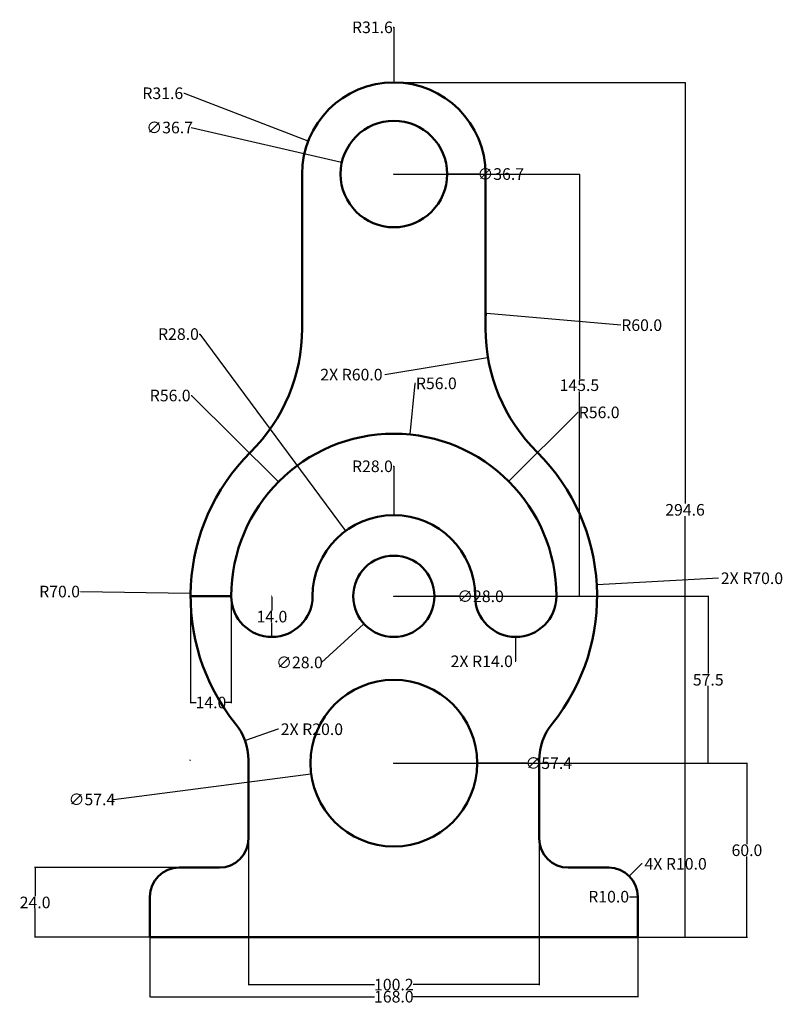
# Model space of a CAD drawing. Units: inches. Extents: x -29 to 234, y -38 to 302.
import ezdxf

# ---------------------------------------------------------------- set-up
doc = ezdxf.new("R2010")
doc.units = ezdxf.units.IN
doc.header["$MEASUREMENT"] = 0
doc.layers.add('M-DIMS', color=2, linetype='Continuous', lineweight=25)
doc.layers.add('M-OUTL', color=7, linetype='Continuous', lineweight=50)
doc.styles.get("Standard").update_dxf_attribs({"font": 'arial.ttf'})
doc.dimstyles.get("Standard").update_dxf_attribs({"dimtxt": 4, "dimasz": 0.18, "dimexe": 0.18, "dimexo": 0.0625, "dimgap": 0.09, "dimtad": 0, "dimtih": 1, "dimtoh": 1, "dimdec": 1, "dimzin": 0, "dimdsep": 46, "dimtxsty": 'Standard', "dimcen": 0.09, "dimadec": 0, "dimazin": 0, "dimtfac": 1, "dimtdec": 1, "dimtofl": 0, "dimtmove": 0, "dimatfit": 3, "dimfxl": 1, "dimtolj": 1, "dimtzin": 0, "dimarcsym": 0})

# ---------------------------------------------------------------- blocks, each defined once
blk = doc.blocks.new('*D1')
at = {"layer": 'Defpoints', "color": 0, "transparency": 16777216}
for p in [(100.04, 45.32), (100.04, -14.68), (221.66, -14.68)]:
    blk.add_point(p, dxfattribs=at)
at = {"layer": 'M-DIMS', "color": 0, "lineweight": -2, "transparency": 16777216}
for p, q in [((100.1, 45.32), (221.84, 45.32)), ((221.66, 45.14), (221.66, 17.46)), ((221.66, -14.5), (221.66, 13.19)), ((100.1, -14.68), (221.84, -14.68))]:
    blk.add_line(p, q, dxfattribs=at)
at = {"layer": 'M-DIMS', "color": 0, "transparency": 16777216}
for points in [[(221.63, 45.14), (221.69, 45.14), (221.66, 45.32)], [(221.63, -14.5), (221.69, -14.5), (221.66, -14.68)]]:
    blk.add_solid(points, dxfattribs=at)
at = {"layer": 'M-DIMS', "color": 0, "transparency": 16777216, "insert": (221.66, 15.32), "char_height": 4, "attachment_point": 5}
blk.add_mtext('\\A1;60.0', dxfattribs=at)
blk = doc.blocks.new('*D2')
at = {"layer": 'Defpoints', "color": 0, "transparency": 16777216}
for p in [(100.04, 102.82), (100.04, 45.32), (208.33, 45.32)]:
    blk.add_point(p, dxfattribs=at)
at = {"layer": 'M-DIMS', "color": 0, "lineweight": -2, "transparency": 16777216}
for p, q in [((100.1, 102.82), (208.51, 102.82)), ((208.33, 102.64), (208.33, 76.2)), ((208.33, 45.5), (208.33, 71.95)), ((100.1, 45.32), (208.51, 45.32))]:
    blk.add_line(p, q, dxfattribs=at)
at = {"layer": 'M-DIMS', "color": 0, "transparency": 16777216}
for points in [[(208.3, 102.64), (208.36, 102.64), (208.33, 102.82)], [(208.3, 45.5), (208.36, 45.5), (208.33, 45.32)]]:
    blk.add_solid(points, dxfattribs=at)
at = {"layer": 'M-DIMS', "color": 0, "transparency": 16777216, "insert": (208.33, 74.07), "char_height": 4, "attachment_point": 5}
blk.add_mtext('\\A1;57.5', dxfattribs=at)
blk = doc.blocks.new('*D3')
at = {"layer": 'Defpoints', "color": 0, "transparency": 16777216}
for p in [(100.04, 248.32), (100.04, 102.82), (163.95, 102.82)]:
    blk.add_point(p, dxfattribs=at)
at = {"layer": 'M-DIMS', "color": 0, "lineweight": -2, "transparency": 16777216}
for p, q in [((100.1, 248.32), (164.13, 248.32)), ((163.95, 248.14), (163.95, 177.71)), ((163.95, 103), (163.95, 173.44)), ((100.1, 102.82), (164.13, 102.82))]:
    blk.add_line(p, q, dxfattribs=at)
at = {"layer": 'M-DIMS', "color": 0, "transparency": 16777216}
for points in [[(163.92, 248.14), (163.98, 248.14), (163.95, 248.32)], [(163.92, 103), (163.98, 103), (163.95, 102.82)]]:
    blk.add_solid(points, dxfattribs=at)
at = {"layer": 'M-DIMS', "color": 0, "transparency": 16777216, "insert": (163.95, 175.57), "char_height": 4, "attachment_point": 5}
blk.add_mtext('\\A1;145.5', dxfattribs=at)
blk = doc.blocks.new('*D4')
at = {"layer": 'Defpoints', "color": 0, "transparency": 16777216}
for p in [(128.5, 49.01), (71.57, 41.64)]:
    blk.add_point(p, dxfattribs=at)
at = {"layer": 'M-DIMS', "color": 0, "lineweight": -2, "transparency": 16777216}
for p, q in [((99.95, 45.32), (100.13, 45.32)), ((100.04, 45.23), (100.04, 45.41)), ((3.49, 32.83), (71.4, 41.62))]:
    blk.add_line(p, q, dxfattribs=at)
at = {"layer": 'M-DIMS', "color": 0, "transparency": 16777216}
blk.add_solid([(71.39, 41.65), (71.4, 41.59), (71.57, 41.64)], dxfattribs=at)
at = {"layer": 'M-DIMS', "color": 0, "transparency": 16777216, "insert": (-3.96, 32.83), "char_height": 4, "attachment_point": 5}
blk.add_mtext('\\A1;∅57.4', dxfattribs=at)
blk = doc.blocks.new('*D5')
at = {"layer": 'Defpoints', "color": 0, "transparency": 16777216}
for p in [(60.3, 142.29), (100.04, 102.82)]:
    blk.add_point(p, dxfattribs=at)
at = {"layer": 'M-DIMS', "color": 0, "lineweight": -2, "transparency": 16777216}
for p, q in [((30.19, 172.01), (30.37, 172.01)), ((30.37, 172.01), (60.18, 142.41)), ((99.95, 102.82), (100.13, 102.82)), ((100.04, 102.73), (100.04, 102.91))]:
    blk.add_line(p, q, dxfattribs=at)
at = {"layer": 'M-DIMS', "color": 0, "transparency": 16777216}
blk.add_solid([(60.2, 142.44), (60.16, 142.39), (60.3, 142.29)], dxfattribs=at)
at = {"layer": 'M-DIMS', "color": 0, "transparency": 16777216, "insert": (23, 172.01), "char_height": 4, "attachment_point": 5}
blk.add_mtext('\\A1;R56.0', dxfattribs=at)
blk = doc.blocks.new('*D6')
at = {"layer": 'Defpoints', "color": 0, "transparency": 16777216}
for p in [(83.39, 125.34), (100.04, 102.82)]:
    blk.add_point(p, dxfattribs=at)
at = {"layer": 'M-DIMS', "color": 0, "lineweight": -2, "transparency": 16777216}
for p, q in [((33.04, 193.18), (33.22, 193.18)), ((33.22, 193.18), (83.28, 125.48)), ((99.95, 102.82), (100.13, 102.82)), ((100.04, 102.73), (100.04, 102.91))]:
    blk.add_line(p, q, dxfattribs=at)
at = {"layer": 'M-DIMS', "color": 0, "transparency": 16777216}
blk.add_solid([(83.31, 125.5), (83.26, 125.46), (83.39, 125.34)], dxfattribs=at)
at = {"layer": 'M-DIMS', "color": 0, "transparency": 16777216, "insert": (25.85, 193.18), "char_height": 4, "attachment_point": 5}
blk.add_mtext('\\A1;R28.0', dxfattribs=at)
blk = doc.blocks.new('*D7')
at = {"layer": 'Defpoints', "color": 0, "transparency": 16777216}
for p in [(58.04, 102.82), (58.04, 88.82), (58.04, 88.82)]:
    blk.add_point(p, dxfattribs=at)
at = {"layer": 'M-DIMS', "color": 0, "lineweight": -2, "transparency": 16777216}
for p, q in [((57.97, 102.82), (57.86, 102.82)), ((58.04, 102.64), (58.04, 97.96)), ((58.04, 89), (58.04, 93.69)), ((57.97, 88.82), (57.86, 88.82))]:
    blk.add_line(p, q, dxfattribs=at)
at = {"layer": 'M-DIMS', "color": 0, "transparency": 16777216}
for points in [[(58.01, 102.64), (58.07, 102.64), (58.04, 102.82)], [(58.01, 89), (58.07, 89), (58.04, 88.82)]]:
    blk.add_solid(points, dxfattribs=at)
at = {"layer": 'M-DIMS', "color": 0, "transparency": 16777216, "insert": (58.04, 95.82), "char_height": 4, "attachment_point": 5}
blk.add_mtext('\\A1;14.0', dxfattribs=at)
blk = doc.blocks.new('*D8')
at = {"layer": 'Defpoints', "color": 0, "transparency": 16777216}
for p in [(110.36, 112.28), (89.72, 93.37)]:
    blk.add_point(p, dxfattribs=at)
at = {"layer": 'M-DIMS', "color": 0, "lineweight": -2, "transparency": 16777216}
for p, q in [((99.95, 102.82), (100.13, 102.82)), ((100.04, 102.73), (100.04, 102.91)), ((75.17, 80.04), (89.58, 93.24)), ((74.99, 80.04), (75.17, 80.04))]:
    blk.add_line(p, q, dxfattribs=at)
at = {"layer": 'M-DIMS', "color": 0, "transparency": 16777216}
blk.add_solid([(89.56, 93.27), (89.6, 93.22), (89.72, 93.37)], dxfattribs=at)
at = {"layer": 'M-DIMS', "color": 0, "transparency": 16777216, "insert": (67.54, 80.04), "char_height": 4, "attachment_point": 5}
blk.add_mtext('\\A1;∅28.0', dxfattribs=at)
blk = doc.blocks.new('*D9')
at = {"layer": 'Defpoints', "color": 0, "transparency": 16777216}
for p in [(30.05, 103.88), (100.04, 102.82)]:
    blk.add_point(p, dxfattribs=at)
at = {"layer": 'M-DIMS', "color": 0, "lineweight": -2, "transparency": 16777216}
for p, q in [((-7.91, 104.46), (29.87, 103.89)), ((99.95, 102.82), (100.13, 102.82)), ((100.04, 102.73), (100.04, 102.91))]:
    blk.add_line(p, q, dxfattribs=at)
at = {"layer": 'M-DIMS', "color": 0, "transparency": 16777216}
blk.add_solid([(29.87, 103.92), (29.86, 103.86), (30.05, 103.88)], dxfattribs=at)
at = {"layer": 'M-DIMS', "color": 0, "transparency": 16777216, "insert": (-15.1, 104.46), "char_height": 4, "attachment_point": 5}
blk.add_mtext('\\A1;R70.0', dxfattribs=at)
blk = doc.blocks.new('*D10')
at = {"layer": 'Defpoints', "color": 0, "transparency": 16777216}
for p in [(82.15, 252.43), (117.92, 244.21)]:
    blk.add_point(p, dxfattribs=at)
at = {"layer": 'M-DIMS', "color": 0, "lineweight": -2, "transparency": 16777216}
for p, q in [((30.28, 264.35), (81.98, 252.47)), ((99.95, 248.32), (100.13, 248.32)), ((100.04, 248.23), (100.04, 248.41))]:
    blk.add_line(p, q, dxfattribs=at)
at = {"layer": 'M-DIMS', "color": 0, "transparency": 16777216}
blk.add_solid([(81.98, 252.5), (81.97, 252.44), (82.15, 252.43)], dxfattribs=at)
at = {"layer": 'M-DIMS', "color": 0, "transparency": 16777216, "insert": (22.82, 264.35), "char_height": 4, "attachment_point": 5}
blk.add_mtext('\\A1;∅36.7', dxfattribs=at)
blk = doc.blocks.new('*D11')
at = {"layer": 'Defpoints', "color": 0, "transparency": 16777216}
for p in [(70.55, 259.69), (100.04, 248.32)]:
    blk.add_point(p, dxfattribs=at)
at = {"layer": 'M-DIMS', "color": 0, "lineweight": -2, "transparency": 16777216}
for p, q in [((27.65, 276.16), (27.83, 276.16)), ((27.83, 276.16), (70.39, 259.76)), ((99.95, 248.32), (100.13, 248.32)), ((100.04, 248.23), (100.04, 248.41))]:
    blk.add_line(p, q, dxfattribs=at)
at = {"layer": 'M-DIMS', "color": 0, "transparency": 16777216}
blk.add_solid([(70.4, 259.79), (70.37, 259.73), (70.55, 259.69)], dxfattribs=at)
at = {"layer": 'M-DIMS', "color": 0, "transparency": 16777216, "insert": (20.46, 276.16), "char_height": 4, "attachment_point": 5}
blk.add_mtext('\\A1;R31.6', dxfattribs=at)
blk = doc.blocks.new('*D12')
at = {"layer": 'Defpoints', "color": 0, "transparency": 16777216}
for p in [(131.87, 200.31), (191.64, 195.07)]:
    blk.add_point(p, dxfattribs=at)
at = {"layer": 'M-DIMS', "color": 0, "lineweight": -2, "transparency": 16777216}
blk.add_line((178.22, 196.25), (132.05, 200.29), dxfattribs=at)
blk.add_arc((191.64, 195.07), 60, 174.821, 179.9403, dxfattribs=at)
at = {"layer": 'M-DIMS', "color": 0, "transparency": 16777216}
blk.add_solid([(132.05, 200.32), (132.04, 200.26), (131.87, 200.31)], dxfattribs=at)
at = {"layer": 'M-DIMS', "color": 0, "transparency": 16777216, "insert": (185.41, 196.25), "char_height": 4, "attachment_point": 5}
blk.add_mtext('\\A1;R60.0', dxfattribs=at)
blk = doc.blocks.new('*D13')
at = {"layer": 'Defpoints', "color": 0, "transparency": 16777216}
for p in [(16.04, -14.68), (184.04, -14.68), (184.04, -35.15)]:
    blk.add_point(p, dxfattribs=at)
at = {"layer": 'M-DIMS', "color": 0, "lineweight": -2, "transparency": 16777216}
for p, q in [((16.04, -14.74), (16.04, -35.33)), ((184.04, -14.74), (184.04, -35.33)), ((16.22, -35.15), (93.39, -35.15)), ((183.86, -35.15), (106.68, -35.15))]:
    blk.add_line(p, q, dxfattribs=at)
at = {"layer": 'M-DIMS', "color": 0, "transparency": 16777216}
for points in [[(16.22, -35.12), (16.22, -35.18), (16.04, -35.15)], [(183.86, -35.12), (183.86, -35.18), (184.04, -35.15)]]:
    blk.add_solid(points, dxfattribs=at)
at = {"layer": 'M-DIMS', "color": 0, "transparency": 16777216, "insert": (100.04, -35.15), "char_height": 4, "attachment_point": 5}
blk.add_mtext('\\A1;168.0', dxfattribs=at)
blk = doc.blocks.new('*D14')
at = {"layer": 'Defpoints', "color": 0, "transparency": 16777216}
for p in [(32.99, 9.32), (-23.53, -14.68), (16.04, -14.68)]:
    blk.add_point(p, dxfattribs=at)
at = {"layer": 'M-DIMS', "color": 0, "lineweight": -2, "transparency": 16777216}
for p, q in [((32.92, 9.32), (-23.71, 9.32)), ((-23.53, 9.14), (-23.53, -0.54)), ((-23.53, -14.5), (-23.53, -4.81)), ((15.97, -14.68), (-23.71, -14.68))]:
    blk.add_line(p, q, dxfattribs=at)
at = {"layer": 'M-DIMS', "color": 0, "transparency": 16777216}
for points in [[(-23.56, 9.14), (-23.5, 9.14), (-23.53, 9.32)], [(-23.56, -14.5), (-23.5, -14.5), (-23.53, -14.68)]]:
    blk.add_solid(points, dxfattribs=at)
at = {"layer": 'M-DIMS', "color": 0, "transparency": 16777216, "insert": (-23.53, -2.68), "char_height": 4, "attachment_point": 5}
blk.add_mtext('\\A1;24.0', dxfattribs=at)
blk = doc.blocks.new('*D15')
at = {"layer": 'Defpoints', "color": 0, "transparency": 16777216}
for p in [(174.04, -0.68), (184.04, -0.68)]:
    blk.add_point(p, dxfattribs=at)
at = {"layer": 'M-DIMS', "color": 0, "lineweight": -2, "transparency": 16777216}
blk.add_line((181.23, -0.68), (183.86, -0.68), dxfattribs=at)
blk.add_arc((174.04, -0.68), 10, 358.9687, 359.6419, dxfattribs=at)
at = {"layer": 'M-DIMS', "color": 0, "transparency": 16777216}
blk.add_solid([(183.86, -0.65), (183.86, -0.71), (184.04, -0.68)], dxfattribs=at)
at = {"layer": 'M-DIMS', "color": 0, "transparency": 16777216, "insert": (174.04, -0.68), "char_height": 4, "attachment_point": 5}
blk.add_mtext('\\A1;R10.0', dxfattribs=at)
blk = doc.blocks.new('*D16')
at = {"layer": 'Defpoints', "color": 0, "transparency": 16777216}
for p in [(105.55, 158.55), (100.04, 102.82)]:
    blk.add_point(p, dxfattribs=at)
at = {"layer": 'M-DIMS', "color": 0, "lineweight": -2, "transparency": 16777216}
for p, q in [((107.3, 176.19), (105.57, 158.73)), ((107.48, 176.19), (107.3, 176.19)), ((99.95, 102.82), (100.13, 102.82)), ((100.04, 102.73), (100.04, 102.91))]:
    blk.add_line(p, q, dxfattribs=at)
at = {"layer": 'M-DIMS', "color": 0, "transparency": 16777216}
blk.add_solid([(105.54, 158.73), (105.6, 158.73), (105.55, 158.55)], dxfattribs=at)
at = {"layer": 'M-DIMS', "color": 0, "transparency": 16777216, "insert": (114.67, 176.19), "char_height": 4, "attachment_point": 5}
blk.add_mtext('\\A1;R56.0', dxfattribs=at)
blk = doc.blocks.new('*D17')
at = {"layer": 'Defpoints', "color": 0, "transparency": 16777216}
for p in [(30.04, 102.82), (44.04, 102.82), (30.04, 66.23)]:
    blk.add_point(p, dxfattribs=at)
at = {"layer": 'M-DIMS', "color": 0, "lineweight": -2, "transparency": 16777216}
for p, q in [((30.04, 102.76), (30.04, 66.05)), ((44.04, 102.76), (44.04, 66.05)), ((30.22, 66.23), (31.95, 66.23)), ((43.86, 66.23), (42.13, 66.23))]:
    blk.add_line(p, q, dxfattribs=at)
at = {"layer": 'M-DIMS', "color": 0, "transparency": 16777216}
for points in [[(30.22, 66.26), (30.22, 66.2), (30.04, 66.23)], [(43.86, 66.26), (43.86, 66.2), (44.04, 66.23)]]:
    blk.add_solid(points, dxfattribs=at)
at = {"layer": 'M-DIMS', "color": 0, "transparency": 16777216, "insert": (37.04, 66.23), "char_height": 4, "attachment_point": 5}
blk.add_mtext('\\A1;14.0', dxfattribs=at)
blk = doc.blocks.new('*D18')
at = {"layer": 'Defpoints', "color": 0, "transparency": 16777216}
for p in [(100.04, 279.92), (200.34, 279.92), (184.04, -14.68)]:
    blk.add_point(p, dxfattribs=at)
at = {"layer": 'M-DIMS', "color": 0, "lineweight": -2, "transparency": 16777216}
for p, q in [((100.1, 279.92), (200.52, 279.92)), ((200.34, 279.74), (200.34, 134.76)), ((200.34, -14.5), (200.34, 130.49)), ((184.1, -14.68), (200.52, -14.68))]:
    blk.add_line(p, q, dxfattribs=at)
at = {"layer": 'M-DIMS', "color": 0, "transparency": 16777216}
for points in [[(200.31, 279.74), (200.37, 279.74), (200.34, 279.92)], [(200.31, -14.5), (200.37, -14.5), (200.34, -14.68)]]:
    blk.add_solid(points, dxfattribs=at)
at = {"layer": 'M-DIMS', "color": 0, "transparency": 16777216, "insert": (200.34, 132.62), "char_height": 4, "attachment_point": 5}
blk.add_mtext('\\A1;294.6', dxfattribs=at)
blk = doc.blocks.new('*D19')
at = {"layer": 'Defpoints', "color": 0, "transparency": 16777216}
for p in [(49.94, 19.32), (150.14, 19.32), (150.14, -30.98)]:
    blk.add_point(p, dxfattribs=at)
at = {"layer": 'M-DIMS', "color": 0, "lineweight": -2, "transparency": 16777216}
for p, q in [((49.94, 19.26), (49.94, -31.16)), ((150.14, 19.26), (150.14, -31.16)), ((50.12, -30.98), (93.41, -30.98)), ((149.96, -30.98), (106.67, -30.98))]:
    blk.add_line(p, q, dxfattribs=at)
at = {"layer": 'M-DIMS', "color": 0, "transparency": 16777216}
for points in [[(50.12, -30.95), (50.12, -31.01), (49.94, -30.98)], [(149.96, -30.95), (149.96, -31.01), (150.14, -30.98)]]:
    blk.add_solid(points, dxfattribs=at)
at = {"layer": 'M-DIMS', "color": 0, "transparency": 16777216, "insert": (100.04, -30.98), "char_height": 4, "attachment_point": 5}
blk.add_mtext('\\A1;100.2', dxfattribs=at)
blk = doc.blocks.new('*D20')
at = {"layer": 'Defpoints', "color": 0, "transparency": 16777216}
for p in [(169.93, 106.71), (100.04, 102.82)]:
    blk.add_point(p, dxfattribs=at)
at = {"layer": 'M-DIMS', "color": 0, "lineweight": -2, "transparency": 16777216}
for p, q in [((211.86, 109.04), (170.11, 106.72)), ((99.95, 102.82), (100.13, 102.82)), ((100.04, 102.73), (100.04, 102.91))]:
    blk.add_line(p, q, dxfattribs=at)
at = {"layer": 'M-DIMS', "color": 0, "transparency": 16777216}
blk.add_solid([(170.11, 106.75), (170.11, 106.69), (169.93, 106.71)], dxfattribs=at)
at = {"layer": 'M-DIMS', "color": 0, "transparency": 16777216, "insert": (223.39, 109.04), "char_height": 4, "attachment_point": 5}
blk.add_mtext('\\A1;2X R70.0', dxfattribs=at)
blk = doc.blocks.new('*D21')
at = {"layer": 'Defpoints', "color": 0, "transparency": 16777216}
for p in [(139.63, 142.43), (100.04, 102.82)]:
    blk.add_point(p, dxfattribs=at)
at = {"layer": 'M-DIMS', "color": 0, "lineweight": -2, "transparency": 16777216}
for p, q in [((163.38, 166.19), (139.76, 142.56)), ((163.56, 166.19), (163.38, 166.19)), ((99.95, 102.82), (100.13, 102.82)), ((100.04, 102.73), (100.04, 102.91))]:
    blk.add_line(p, q, dxfattribs=at)
at = {"layer": 'M-DIMS', "color": 0, "transparency": 16777216}
blk.add_solid([(139.73, 142.58), (139.78, 142.53), (139.63, 142.43)], dxfattribs=at)
at = {"layer": 'M-DIMS', "color": 0, "transparency": 16777216, "insert": (170.76, 166.19), "char_height": 4, "attachment_point": 5}
blk.add_mtext('\\A1;R56.0', dxfattribs=at)
blk = doc.blocks.new('*D22')
at = {"layer": 'Defpoints', "color": 0, "transparency": 16777216}
for p in [(100.04, 279.92), (100.04, 248.32)]:
    blk.add_point(p, dxfattribs=at)
at = {"layer": 'M-DIMS', "color": 0, "lineweight": -2, "transparency": 16777216}
for p, q in [((99.86, 298.88), (100.04, 298.88)), ((100.04, 298.88), (100.04, 280.1)), ((99.95, 248.32), (100.13, 248.32)), ((100.04, 248.23), (100.04, 248.41))]:
    blk.add_line(p, q, dxfattribs=at)
at = {"layer": 'M-DIMS', "color": 0, "transparency": 16777216}
blk.add_solid([(100.07, 280.1), (100.01, 280.1), (100.04, 279.92)], dxfattribs=at)
at = {"layer": 'M-DIMS', "color": 0, "transparency": 16777216, "insert": (92.66, 298.88), "char_height": 4, "attachment_point": 5}
blk.add_mtext('\\A1;R31.6', dxfattribs=at)
blk = doc.blocks.new('*D23')
at = {"layer": 'Defpoints', "color": 0, "transparency": 16777216}
for p in [(71.34, 45.32), (128.74, 45.32)]:
    blk.add_point(p, dxfattribs=at)
at = {"layer": 'M-DIMS', "color": 0, "lineweight": -2, "transparency": 16777216}
for p, q in [((99.95, 45.32), (100.13, 45.32)), ((100.04, 45.23), (100.04, 45.41)), ((145.96, 45.32), (128.92, 45.32))]:
    blk.add_line(p, q, dxfattribs=at)
at = {"layer": 'M-DIMS', "color": 0, "transparency": 16777216}
blk.add_solid([(128.92, 45.35), (128.92, 45.29), (128.74, 45.32)], dxfattribs=at)
at = {"layer": 'M-DIMS', "color": 0, "transparency": 16777216, "insert": (153.41, 45.32), "char_height": 4, "attachment_point": 5}
blk.add_mtext('\\A1;∅57.4', dxfattribs=at)
blk = doc.blocks.new('*D24')
at = {"layer": 'Defpoints', "color": 0, "transparency": 16777216}
for p in [(100.04, 130.82), (100.04, 102.82)]:
    blk.add_point(p, dxfattribs=at)
at = {"layer": 'M-DIMS', "color": 0, "lineweight": -2, "transparency": 16777216}
for p, q in [((99.86, 147.62), (100.04, 147.62)), ((100.04, 147.62), (100.04, 131)), ((99.95, 102.82), (100.13, 102.82)), ((100.04, 102.73), (100.04, 102.91))]:
    blk.add_line(p, q, dxfattribs=at)
at = {"layer": 'M-DIMS', "color": 0, "transparency": 16777216}
blk.add_solid([(100.07, 131), (100.01, 131), (100.04, 130.82)], dxfattribs=at)
at = {"layer": 'M-DIMS', "color": 0, "transparency": 16777216, "insert": (92.66, 147.62), "char_height": 4, "attachment_point": 5}
blk.add_mtext('\\A1;R28.0', dxfattribs=at)
blk = doc.blocks.new('*D25')
at = {"layer": 'Defpoints', "color": 0, "transparency": 16777216}
for p in [(48.8, 53.03), (29.94, 46.38)]:
    blk.add_point(p, dxfattribs=at)
at = {"layer": 'M-DIMS', "color": 0, "lineweight": -2, "transparency": 16777216}
for p, q in [((60.12, 57.02), (48.97, 53.09)), ((60.3, 57.02), (60.12, 57.02)), ((29.85, 46.38), (30.03, 46.38)), ((29.94, 46.29), (29.94, 46.47))]:
    blk.add_line(p, q, dxfattribs=at)
at = {"layer": 'M-DIMS', "color": 0, "transparency": 16777216}
blk.add_solid([(48.96, 53.12), (48.98, 53.06), (48.8, 53.03)], dxfattribs=at)
at = {"layer": 'M-DIMS', "color": 0, "transparency": 16777216, "insert": (71.82, 57.02), "char_height": 4, "attachment_point": 5}
blk.add_mtext('\\A1;2X R20.0', dxfattribs=at)
blk = doc.blocks.new('*D26')
at = {"layer": 'Defpoints', "color": 0, "transparency": 16777216}
for p in [(81.69, 248.32), (118.39, 248.32)]:
    blk.add_point(p, dxfattribs=at)
at = {"layer": 'M-DIMS', "color": 0, "lineweight": -2, "transparency": 16777216}
for p, q in [((99.95, 248.32), (100.13, 248.32)), ((100.04, 248.23), (100.04, 248.41)), ((129.4, 248.32), (118.57, 248.32))]:
    blk.add_line(p, q, dxfattribs=at)
at = {"layer": 'M-DIMS', "color": 0, "transparency": 16777216}
blk.add_solid([(118.57, 248.35), (118.57, 248.29), (118.39, 248.32)], dxfattribs=at)
at = {"layer": 'M-DIMS', "color": 0, "transparency": 16777216, "insert": (136.86, 248.32), "char_height": 4, "attachment_point": 5}
blk.add_mtext('\\A1;∅36.7', dxfattribs=at)
blk = doc.blocks.new('*D27')
at = {"layer": 'Defpoints', "color": 0, "transparency": 16777216}
for p in [(86.04, 102.82), (114.04, 102.82)]:
    blk.add_point(p, dxfattribs=at)
at = {"layer": 'M-DIMS', "color": 0, "lineweight": -2, "transparency": 16777216}
for p, q in [((99.95, 102.82), (100.13, 102.82)), ((100.04, 102.73), (100.04, 102.91)), ((122.44, 102.82), (114.22, 102.82))]:
    blk.add_line(p, q, dxfattribs=at)
at = {"layer": 'M-DIMS', "color": 0, "transparency": 16777216}
blk.add_solid([(114.22, 102.85), (114.22, 102.79), (114.04, 102.82)], dxfattribs=at)
at = {"layer": 'M-DIMS', "color": 0, "transparency": 16777216, "insert": (129.89, 102.82), "char_height": 4, "attachment_point": 5}
blk.add_mtext('\\A1;∅28.0', dxfattribs=at)
blk = doc.blocks.new('*D28')
at = {"layer": 'Defpoints', "color": 0, "transparency": 16777216}
for p in [(142.04, 102.82), (142.04, 88.82)]:
    blk.add_point(p, dxfattribs=at)
at = {"layer": 'M-DIMS', "color": 0, "lineweight": -2, "transparency": 16777216}
for p, q in [((141.95, 102.82), (142.13, 102.82)), ((142.04, 102.73), (142.04, 102.91)), ((142.04, 80.42), (142.04, 88.64)), ((141.86, 80.42), (142.04, 80.42))]:
    blk.add_line(p, q, dxfattribs=at)
at = {"layer": 'M-DIMS', "color": 0, "transparency": 16777216}
blk.add_solid([(142.01, 88.64), (142.07, 88.64), (142.04, 88.82)], dxfattribs=at)
at = {"layer": 'M-DIMS', "color": 0, "transparency": 16777216, "insert": (130.33, 80.42), "char_height": 4, "attachment_point": 5}
blk.add_mtext('\\A1;2X R14.0', dxfattribs=at)
blk = doc.blocks.new('*D29')
at = {"layer": 'Defpoints', "color": 0, "transparency": 16777216}
for p in [(181.11, 6.4), (174.04, -0.68)]:
    blk.add_point(p, dxfattribs=at)
at = {"layer": 'M-DIMS', "color": 0, "lineweight": -2, "transparency": 16777216}
for p, q in [((185.35, 10.64), (181.24, 6.52)), ((185.53, 10.64), (185.35, 10.64)), ((173.95, -0.68), (174.13, -0.68)), ((174.04, -0.77), (174.04, -0.59))]:
    blk.add_line(p, q, dxfattribs=at)
at = {"layer": 'M-DIMS', "color": 0, "transparency": 16777216}
blk.add_solid([(181.21, 6.54), (181.26, 6.5), (181.11, 6.4)], dxfattribs=at)
at = {"layer": 'M-DIMS', "color": 0, "transparency": 16777216, "insert": (197.1, 10.64), "char_height": 4, "attachment_point": 5}
blk.add_mtext('\\A1;4X R10.0', dxfattribs=at)
blk = doc.blocks.new('*D30')
at = {"layer": 'Defpoints', "color": 0, "transparency": 16777216}
for p in [(191.64, 195.07), (132.46, 185.16)]:
    blk.add_point(p, dxfattribs=at)
at = {"layer": 'M-DIMS', "color": 0, "lineweight": -2, "transparency": 16777216}
for p, q in [((191.55, 195.07), (191.73, 195.07)), ((191.64, 194.98), (191.64, 195.16)), ((96.96, 179.21), (132.28, 185.13))]:
    blk.add_line(p, q, dxfattribs=at)
at = {"layer": 'M-DIMS', "color": 0, "transparency": 16777216}
blk.add_solid([(132.28, 185.16), (132.29, 185.1), (132.46, 185.16)], dxfattribs=at)
at = {"layer": 'M-DIMS', "color": 0, "transparency": 16777216, "insert": (85.43, 179.21), "char_height": 4, "attachment_point": 5}
blk.add_mtext('\\A1;2X R60.0', dxfattribs=at)

msp = doc.modelspace()

# ---------------------------------------------------------------- linework, layer by layer
at = {"layer": 'M-OUTL'}
for p, q in [((68.44, 248.32), (68.44, 195.07)), ((131.64, 248.32), (131.64, 195.07)), ((44.04, 102.82), (30.04, 102.82)), ((49.94, 45.32), (49.94, 46.38)), ((49.94, 45.32), (49.94, 19.32)), ((150.14, 45.32), (150.14, 46.38)), ((150.14, 45.32), (150.14, 19.32)), ((39.94, 9.32), (26.04, 9.32)), ((160.14, 9.32), (174.04, 9.32)), ((16.04, -14.68), (16.04, -0.68)), ((184.04, -14.68), (184.04, -0.68)), ((16.04, -14.68), (184.04, -14.68))]:
    msp.add_line(p, q, dxfattribs=at)
for centre, radius in [((100.04, 248.32), 18.35), ((100.04, 102.82), 14), ((100.04, 45.32), 28.7)]:
    msp.add_circle(centre, radius, dxfattribs=at)
for centre, radius, start, end in [((100.04, 248.32), 31.6, 0, 180), ((8.44, 195.07), 60, 314.7985, 0), ((191.64, 195.07), 60, 180, 225.2015), ((100.04, 102.82), 56, 0, 180), ((100.04, 102.82), 70, 134.7985, 218.841), ((100.04, 102.82), 70, 321.159, 45.2015), ((100.04, 102.82), 28, 0, 180), ((58.04, 102.82), 14, 180, 0), ((142.04, 102.82), 14, 180, 0), ((29.94, 46.38), 20, 360, 38.841), ((170.14, 46.38), 20, 141.159, 180), ((39.94, 19.32), 10, 270, 0), ((160.14, 19.32), 10, 180, 270), ((26.04, -0.68), 10, 90, 180), ((174.04, -0.68), 10, 0, 90)]:
    msp.add_arc(centre, radius, start, end, dxfattribs=at)

# ---------------------------------------------------------------- dimensions: what is measured, and where the dimension line sits
at = {"layer": 'M-DIMS'}
for center, mpoint, override, picture, middle in [((100.04, 248.32), (100.04, 279.92), {"dimdec": 1, "dimlfac": 1, "dimrnd": 0, "dimzin": 0, "dimdsep": 46, "dimlunit": 2}, '*D22', (92.66, 298.88)), ((100.04, 248.32), (70.55, 259.69), {"dimclrd": 0, "dimclre": 0, "dimclrt": 0}, '*D11', (20.46, 276.16)), ((191.64, 195.07), (131.87, 200.31), {"dimclrd": 0, "dimclre": 0, "dimclrt": 0}, '*D12', (178.22, 196.25)), ((100.04, 102.82), (83.39, 125.34), {"dimclrd": 0, "dimclre": 0, "dimclrt": 0}, '*D6', (25.85, 193.18)), ((100.04, 102.82), (105.55, 158.55), {"dimclrd": 0, "dimclre": 0, "dimclrt": 0}, '*D16', (114.67, 176.19)), ((100.04, 102.82), (60.3, 142.29), {"dimclrd": 0, "dimclre": 0, "dimclrt": 0}, '*D5', (23, 172.01)), ((100.04, 102.82), (139.63, 142.43), {"dimdec": 1, "dimlfac": 1, "dimrnd": 0, "dimzin": 0, "dimdsep": 46, "dimlunit": 2}, '*D21', (170.76, 166.19)), ((100.04, 102.82), (100.04, 130.82), {"dimdec": 1, "dimlfac": 1, "dimrnd": 0, "dimzin": 0, "dimdsep": 46, "dimlunit": 2}, '*D24', (92.66, 147.62)), ((100.04, 102.82), (30.05, 103.88), {"dimclrd": 0, "dimclre": 0, "dimclrt": 0}, '*D9', (-7.91, 104.46)), ((174.04, -0.68), (184.04, -0.68), {"dimclrd": 0, "dimclre": 0, "dimclrt": 0}, '*D15', (174.04, -0.68))]:
    dim = msp.add_radius_dim(center=center, mpoint=mpoint, dimstyle='Standard', override=override, dxfattribs=at)
    dim.commit()
    dim.dimension.update_dxf_attribs({"geometry": picture, "text_midpoint": middle, "dimtype": 164})
for base, p1, p2, override, picture, middle in [((200.34, 279.92), (184.04, -14.68), (100.04, 279.92), {"dimdec": 1, "dimlfac": 1, "dimrnd": 0, "dimzin": 0, "dimdsep": 46, "dimlunit": 2}, '*D18', (200.34, 132.62)), ((163.95, 102.82), (100.04, 248.32), (100.04, 102.82), {"dimclrd": 0, "dimclre": 0, "dimclrt": 0}, '*D3', (163.95, 175.57)), ((58.04, 88.82), (58.04, 102.82), (58.04, 88.82), {"dimclrd": 0, "dimclre": 0, "dimclrt": 0}, '*D7', (58.04, 95.82)), ((208.33, 45.32), (100.04, 102.82), (100.04, 45.32), {"dimclrd": 0, "dimclre": 0, "dimclrt": 0}, '*D2', (208.33, 74.07)), ((221.66, -14.68), (100.04, 45.32), (100.04, -14.68), {"dimclrd": 0, "dimclre": 0, "dimclrt": 0}, '*D1', (221.66, 15.32)), ((-23.53, -14.68), (32.99, 9.32), (16.04, -14.68), {"dimclrd": 0, "dimclre": 0, "dimclrt": 0}, '*D14', (-23.53, -2.68))]:
    dim = msp.add_linear_dim(base=base, p1=p1, p2=p2, angle=90, dimstyle='Standard', override=override, dxfattribs=at)
    dim.commit()
    dim.dimension.update_dxf_attribs({"geometry": picture, "text_midpoint": middle})
for p1, p2, override, picture, middle in [((117.92, 244.21), (82.15, 252.43), {"dimclrd": 0, "dimclre": 0, "dimclrt": 0}, '*D10', (30.28, 264.35)), ((81.69, 248.32), (118.39, 248.32), {"dimdec": 1, "dimlfac": 1, "dimrnd": 0, "dimzin": 0, "dimdsep": 46, "dimlunit": 2}, '*D26', (129.4, 248.32)), ((110.36, 112.28), (89.72, 93.37), {"dimclrd": 0, "dimclre": 0, "dimclrt": 0}, '*D8', (67.54, 80.04)), ((86.04, 102.82), (114.04, 102.82), {"dimdec": 1, "dimlfac": 1, "dimrnd": 0, "dimzin": 0, "dimdsep": 46, "dimlunit": 2}, '*D27', (122.44, 102.82)), ((128.5, 49.01), (71.57, 41.64), {"dimclrd": 0, "dimclre": 0, "dimclrt": 0}, '*D4', (3.49, 32.83)), ((71.34, 45.32), (128.74, 45.32), {"dimdec": 1, "dimlfac": 1, "dimrnd": 0, "dimzin": 0, "dimdsep": 46, "dimlunit": 2}, '*D23', (145.96, 45.32))]:
    dim = msp.add_diameter_dim_2p(p1=p1, p2=p2, dimstyle='Standard', override=override, dxfattribs=at)
    dim.commit()
    dim.dimension.update_dxf_attribs({"geometry": picture, "text_midpoint": middle, "dimtype": 163})
for center, mpoint, text, picture, middle in [((191.64, 195.07), (132.46, 185.16), '2X <>', '*D30', (96.96, 179.21)), ((100.04, 102.82), (169.93, 106.71), '2X <>', '*D20', (211.86, 109.04)), ((142.04, 102.82), (142.04, 88.82), '2X <>', '*D28', (130.33, 80.42)), ((29.94, 46.38), (48.8, 53.03), '2X <>', '*D25', (71.82, 57.02)), ((174.04, -0.68), (181.11, 6.4), '4X <>', '*D29', (197.1, 10.64))]:
    dim = msp.add_radius_dim(center=center, mpoint=mpoint, text=text, dimstyle='Standard', override={"dimdec": 1, "dimlfac": 1, "dimrnd": 0, "dimzin": 0, "dimdsep": 46, "dimlunit": 2}, dxfattribs=at)
    dim.commit()
    dim.dimension.update_dxf_attribs({"geometry": picture, "text_midpoint": middle, "dimtype": 164})
for base, p1, p2, override, picture, middle in [((30.04, 66.23), (44.04, 102.82), (30.04, 102.82), {"dimclrd": 0, "dimclre": 0, "dimclrt": 0}, '*D17', (37.04, 66.23)), ((150.14, -30.98), (49.94, 19.32), (150.14, 19.32), {"dimdec": 1, "dimlfac": 1, "dimrnd": 0, "dimzin": 0, "dimdsep": 46, "dimlunit": 2}, '*D19', (100.04, -30.98)), ((184.04, -35.15), (16.04, -14.68), (184.04, -14.68), {"dimclrd": 0, "dimclre": 0, "dimclrt": 0}, '*D13', (100.04, -35.15))]:
    dim = msp.add_linear_dim(base=base, p1=p1, p2=p2, dimstyle='Standard', override=override, dxfattribs=at)
    dim.commit()
    dim.dimension.update_dxf_attribs({"geometry": picture, "text_midpoint": middle})

doc.saveas('drawing.dxf')
